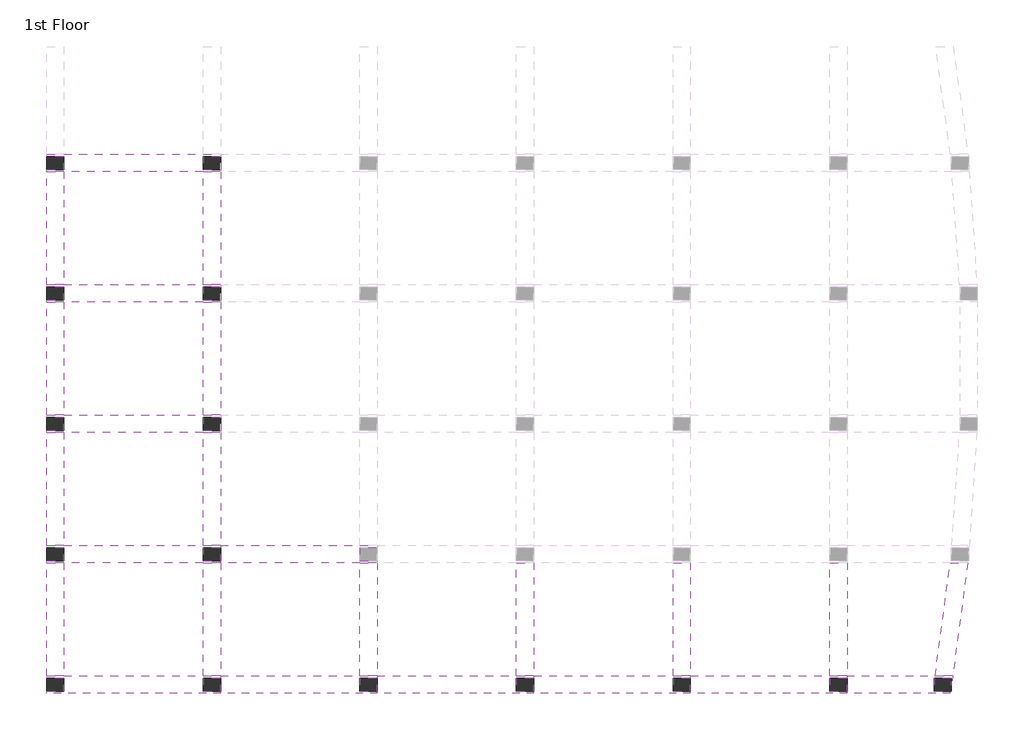
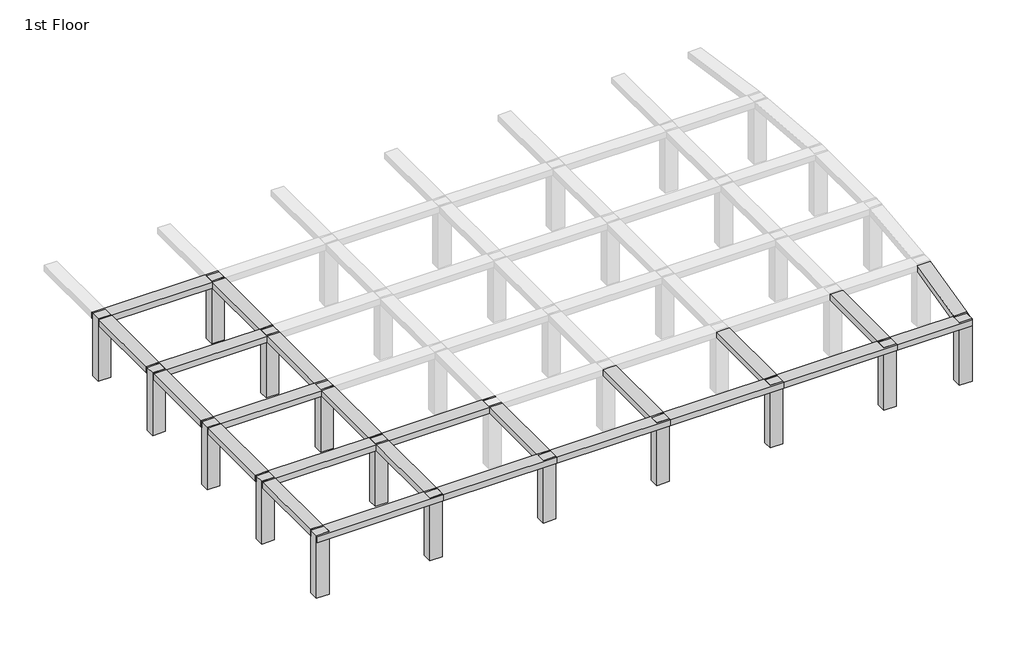
# One storey, part 1 of 3: 24 beams, 15 columns.
"""IFC4 building model written with IfcOpenShell, lengths in millimetres."""

from ifc_helpers import new_model, si_unit, frame, origin, place, context, project, spatial, polyline, outline, extrude, faceted_brep, element, save

model = new_model("IFC4")

# Units and contexts
model_context = context("Model", 3, world=origin())
ifc_project = project(units=[si_unit("LENGTHUNIT", "METRE", prefix="MILLI")], contexts=[model_context])

# Site, building, storey
site = spatial("IfcSite", under=ifc_project)
building = spatial("IfcBuilding", under=site)
storey = spatial("IfcBuildingStorey", under=building, Name="1st Floor", Elevation=3200.4)

# Beams
placement = place(None, origin())
element("IfcBeam", 1, ObjectType="Concrete-Rectangular Beam : 2' x2'", at=placement, inside=storey, context=model_context, shape_type="Brep", body=[
    faceted_brep([(-16619.274232, -2891.2168778, 6400.8), (-17228.874232, -2891.2168778, 6400.8), (-22105.674232, -2891.2168778, 6400.8), (-22715.274232, -2891.2168778, 6400.8), (-22715.274232, -2967.4168778, 6400.8), (-22105.674232, -2967.4168778, 6400.8), (-22105.674232, -3424.6168778, 6400.8), (-22715.274232, -3424.6168778, 6400.8), (-22715.274232, -3500.8168778, 6400.8), (-16619.274232, -3500.8168778, 6400.8), (-16619.274232, -3424.6168778, 6400.8), (-17228.874232, -3424.6168778, 6400.8), (-17228.874232, -2967.4168778, 6400.8), (-16619.274232, -2967.4168778, 6400.8), (-22715.274232, -3500.8168778, 6096.0), (-16619.274232, -3500.8168778, 6096.0), (-22715.274232, -3424.6168778, 6096.0), (-22105.674232, -3424.6168778, 6096.0), (-22105.674232, -2967.4168778, 6096.0), (-22715.274232, -2967.4168778, 6096.0), (-22715.274232, -2891.2168778, 6096.0), (-22105.674232, -2891.2168778, 6096.0), (-17228.874232, -2891.2168778, 6096.0), (-16619.274232, -2891.2168778, 6096.0), (-16619.274232, -2967.4168778, 6096.0), (-17228.874232, -2967.4168778, 6096.0), (-17228.874232, -3424.6168778, 6096.0), (-16619.274232, -3424.6168778, 6096.0)], [[[0, 1, 2, 3, 4, 5, 6, 7, 8, 9, 10, 11, 12, 13]], [[8, 14, 15, 9]], [[15, 14, 16, 17, 18, 19, 20, 21, 22, 23, 24, 25, 26, 27]], [[20, 3, 2, 1, 0, 23, 22, 21]], [[14, 8, 7, 16]], [[9, 15, 27, 10]], [[17, 6, 5, 18]], [[6, 17, 16, 7]], [[18, 5, 4, 19]], [[3, 20, 19, 4]], [[26, 11, 10, 27]], [[11, 26, 25, 12]], [[12, 25, 24, 13]], [[23, 0, 13, 24]]]),
])
element("IfcBeam", 2, ObjectType="Concrete-Rectangular Beam : 2' x2'", at=placement, inside=storey, context=model_context, shape_type="Brep", body=[
    faceted_brep([(-16619.274232, -2891.2168778, 6400.8), (-16619.274232, -2967.4168778, 6400.8), (-16619.274232, -3424.6168778, 6400.8), (-16619.274232, -3500.8168778, 6400.8), (-11132.874232, -3500.8168778, 6400.8), (-11132.874232, -3424.6168778, 6400.8), (-11742.474232, -3424.6168778, 6400.8), (-11742.474232, -2967.4168778, 6400.8), (-11132.874232, -2967.4168778, 6400.8), (-11132.874232, -2891.2168778, 6400.8), (-11742.474232, -2891.2168778, 6400.8), (-11132.874232, -3500.8168778, 6096.0), (-16619.274232, -3500.8168778, 6096.0), (-16619.274232, -3424.6168778, 6096.0), (-16619.274232, -2967.4168778, 6096.0), (-16619.274232, -2891.2168778, 6096.0), (-11742.474232, -2891.2168778, 6096.0), (-11132.874232, -2891.2168778, 6096.0), (-11132.874232, -2967.4168778, 6096.0), (-11742.474232, -2967.4168778, 6096.0), (-11742.474232, -3424.6168778, 6096.0), (-11132.874232, -3424.6168778, 6096.0)], [[[0, 1, 2, 3, 4, 5, 6, 7, 8, 9, 10]], [[11, 4, 3, 12]], [[12, 13, 14, 15, 16, 17, 18, 19, 20, 21, 11]], [[15, 0, 10, 9, 17, 16]], [[3, 2, 1, 0, 15, 14, 13, 12]], [[4, 11, 21, 5]], [[20, 6, 5, 21]], [[6, 20, 19, 7]], [[7, 19, 18, 8]], [[17, 9, 8, 18]]]),
])
element("IfcBeam", 3, ObjectType="Concrete-Rectangular Beam : 2' x2'", at=placement, inside=storey, context=model_context, shape_type="Brep", body=[
    faceted_brep([(-5646.474232, -2891.2168778, 6400.8), (-6256.074232, -2891.2168778, 6400.8), (-11132.874232, -2891.2168778, 6400.8), (-11132.874232, -2967.4168778, 6400.8), (-11132.874232, -3424.6168778, 6400.8), (-11132.874232, -3500.8168778, 6400.8), (-5646.474232, -3500.8168778, 6400.8), (-5646.474232, -3424.6168778, 6400.8), (-6256.074232, -3424.6168778, 6400.8), (-6256.074232, -2967.4168778, 6400.8), (-5646.474232, -2967.4168778, 6400.8), (-5646.474232, -3500.8168778, 6096.0), (-11132.874232, -3500.8168778, 6096.0), (-11132.874232, -3424.6168778, 6096.0), (-11132.874232, -2967.4168778, 6096.0), (-11132.874232, -2891.2168778, 6096.0), (-6256.074232, -2891.2168778, 6096.0), (-5646.474232, -2891.2168778, 6096.0), (-5646.474232, -2967.4168778, 6096.0), (-6256.074232, -2967.4168778, 6096.0), (-6256.074232, -3424.6168778, 6096.0), (-5646.474232, -3424.6168778, 6096.0)], [[[0, 1, 2, 3, 4, 5, 6, 7, 8, 9, 10]], [[11, 6, 5, 12]], [[11, 12, 13, 14, 15, 16, 17, 18, 19, 20, 21]], [[0, 17, 16, 15, 2, 1]], [[6, 11, 21, 7]], [[5, 4, 3, 2, 15, 14, 13, 12]], [[20, 8, 7, 21]], [[8, 20, 19, 9]], [[9, 19, 18, 10]], [[17, 0, 10, 18]]]),
])
element("IfcBeam", 4, ObjectType="Concrete-Rectangular Beam : 2' x2'", at=placement, inside=storey, context=model_context, shape_type="Brep", body=[
    faceted_brep([(-5646.474232, -2891.2168778, 6400.8), (-5646.474232, -2967.4168778, 6400.8), (-5646.474232, -3424.6168778, 6400.8), (-5646.474232, -3500.8168778, 6400.8), (-160.074232, -3500.8168778, 6400.8), (-160.074232, -3424.6168778, 6400.8), (-769.674232, -3424.6168778, 6400.8), (-769.674232, -2967.4168778, 6400.8), (-160.074232, -2967.4168778, 6400.8), (-160.074232, -2891.2168778, 6400.8), (-769.674232, -2891.2168778, 6400.8), (-160.074232, -3500.8168778, 6096.0), (-5646.474232, -3500.8168778, 6096.0), (-5646.474232, -3424.6168778, 6096.0), (-5646.474232, -2967.4168778, 6096.0), (-5646.474232, -2891.2168778, 6096.0), (-769.674232, -2891.2168778, 6096.0), (-160.074232, -2891.2168778, 6096.0), (-160.074232, -2967.4168778, 6096.0), (-769.674232, -2967.4168778, 6096.0), (-769.674232, -3424.6168778, 6096.0), (-160.074232, -3424.6168778, 6096.0)], [[[0, 1, 2, 3, 4, 5, 6, 7, 8, 9, 10]], [[11, 4, 3, 12]], [[12, 13, 14, 15, 16, 17, 18, 19, 20, 21, 11]], [[15, 0, 10, 9, 17, 16]], [[3, 2, 1, 0, 15, 14, 13, 12]], [[4, 11, 21, 5]], [[20, 6, 5, 21]], [[6, 20, 19, 7]], [[7, 19, 18, 8]], [[17, 9, 8, 18]]]),
])
element("IfcBeam", 5, ObjectType="Concrete-Rectangular Beam : 2' x2'", at=placement, inside=storey, context=model_context, shape_type="Brep", body=[
    faceted_brep([(-160.074232, -2891.2168778, 6400.8), (-160.074232, -2967.4168778, 6400.8), (-160.074232, -3424.6168778, 6400.8), (-160.074232, -3500.8168778, 6400.8), (5326.325768, -3500.8168778, 6400.8), (5326.325768, -3424.6168778, 6400.8), (4716.725768, -3424.6168778, 6400.8), (4716.725768, -2967.4168778, 6400.8), (5326.325768, -2967.4168778, 6400.8), (5326.325768, -2891.2168778, 6400.8), (4716.725768, -2891.2168778, 6400.8), (5326.325768, -3500.8168778, 6096.0), (-160.074232, -3500.8168778, 6096.0), (-160.074232, -3424.6168778, 6096.0), (-160.074232, -2967.4168778, 6096.0), (-160.074232, -2891.2168778, 6096.0), (4716.725768, -2891.2168778, 6096.0), (5326.325768, -2891.2168778, 6096.0), (5326.325768, -2967.4168778, 6096.0), (4716.725768, -2967.4168778, 6096.0), (4716.725768, -3424.6168778, 6096.0), (5326.325768, -3424.6168778, 6096.0)], [[[0, 1, 2, 3, 4, 5, 6, 7, 8, 9, 10]], [[11, 4, 3, 12]], [[12, 13, 14, 15, 16, 17, 18, 19, 20, 21, 11]], [[15, 0, 10, 9, 17, 16]], [[3, 2, 1, 0, 15, 14, 13, 12]], [[4, 11, 21, 5]], [[20, 6, 5, 21]], [[6, 20, 19, 7]], [[7, 19, 18, 8]], [[17, 9, 8, 18]]]),
])
element("IfcBeam", 6, ObjectType="Concrete-Rectangular Beam : 2' x2'", at=placement, inside=storey, context=model_context, shape_type="Brep", body=[
    faceted_brep([(9027.2344863, -2891.2168778, 6400.8), (8412.2463849, -2891.2168778, 6400.8), (5326.325768, -2891.2168778, 6400.8), (5326.325768, -2967.4168778, 6400.8), (5326.325768, -3424.6168778, 6400.8), (5326.325768, -3500.8168778, 6400.8), (8946.005151, -3500.8168778, 6400.8), (8956.158818, -3424.6168778, 6400.8), (8374.325768, -3424.6168778, 6400.8), (8374.325768, -2967.4168778, 6400.8), (8983.925768, -2967.4168778, 6400.8), (8983.925768, -3216.2348608, 6400.8), (8946.005151, -3500.8168778, 6096.0), (5326.325768, -3500.8168778, 6096.0), (5326.325768, -3424.6168778, 6096.0), (5326.325768, -2967.4168778, 6096.0), (5326.325768, -2891.2168778, 6096.0), (8412.2463849, -2891.2168778, 6096.0), (9027.2344863, -2891.2168778, 6096.0), (8983.925768, -3216.2348608, 6096.0), (8983.925768, -2967.4168778, 6096.0), (8374.325768, -2967.4168778, 6096.0), (8374.325768, -3424.6168778, 6096.0), (8956.158818, -3424.6168778, 6096.0)], [[[0, 1, 2, 3, 4, 5, 6, 7, 8, 9, 10, 11]], [[12, 6, 5, 13]], [[12, 13, 14, 15, 16, 17, 18, 19, 20, 21, 22, 23]], [[0, 18, 17, 16, 2, 1]], [[6, 12, 23, 7]], [[5, 4, 3, 2, 16, 15, 14, 13]], [[10, 20, 19, 11]], [[22, 8, 7, 23]], [[8, 22, 21, 9]], [[9, 21, 20, 10]], [[18, 0, 11, 19]]]),
])
element("IfcBeam", 7, ObjectType="Concrete-Rectangular Beam : 2' x2'", at=placement, inside=storey, context=model_context, shape_type="Brep", body=[
    faceted_brep([(-16619.274232, 1680.7831222, 6400.8), (-17228.874232, 1680.7831222, 6400.8), (-22105.674232, 1680.7831222, 6400.8), (-22715.274232, 1680.7831222, 6400.8), (-22715.274232, 1604.5831222, 6400.8), (-22105.674232, 1604.5831222, 6400.8), (-22105.674232, 1147.3831222, 6400.8), (-22715.274232, 1147.3831222, 6400.8), (-22715.274232, 1071.1831222, 6400.8), (-22105.674232, 1071.1831222, 6400.8), (-17228.874232, 1071.1831222, 6400.8), (-16619.274232, 1071.1831222, 6400.8), (-16619.274232, 1147.3831222, 6400.8), (-17228.874232, 1147.3831222, 6400.8), (-17228.874232, 1604.5831222, 6400.8), (-16619.274232, 1604.5831222, 6400.8), (-22715.274232, 1071.1831222, 6096.0), (-22105.674232, 1071.1831222, 6096.0), (-17228.874232, 1071.1831222, 6096.0), (-16619.274232, 1071.1831222, 6096.0), (-22715.274232, 1147.3831222, 6096.0), (-22105.674232, 1147.3831222, 6096.0), (-22105.674232, 1604.5831222, 6096.0), (-22715.274232, 1604.5831222, 6096.0), (-22715.274232, 1680.7831222, 6096.0), (-22105.674232, 1680.7831222, 6096.0), (-17228.874232, 1680.7831222, 6096.0), (-16619.274232, 1680.7831222, 6096.0), (-16619.274232, 1604.5831222, 6096.0), (-17228.874232, 1604.5831222, 6096.0), (-17228.874232, 1147.3831222, 6096.0), (-16619.274232, 1147.3831222, 6096.0)], [[[0, 1, 2, 3, 4, 5, 6, 7, 8, 9, 10, 11, 12, 13, 14, 15]], [[8, 16, 17, 18, 19, 11, 10, 9]], [[19, 18, 17, 16, 20, 21, 22, 23, 24, 25, 26, 27, 28, 29, 30, 31]], [[24, 3, 2, 1, 0, 27, 26, 25]], [[16, 8, 7, 20]], [[11, 19, 31, 12]], [[21, 6, 5, 22]], [[6, 21, 20, 7]], [[22, 5, 4, 23]], [[3, 24, 23, 4]], [[30, 13, 12, 31]], [[13, 30, 29, 14]], [[14, 29, 28, 15]], [[27, 0, 15, 28]]]),
])
element("IfcBeam", 8, ObjectType="Concrete-Rectangular Beam : 2' x2'", at=placement, inside=storey, context=model_context, shape_type="Brep", body=[
    faceted_brep([(-16619.274232, 1680.7831222, 6400.8), (-16619.274232, 1604.5831222, 6400.8), (-16619.274232, 1147.3831222, 6400.8), (-16619.274232, 1071.1831222, 6400.8), (-11742.474232, 1071.1831222, 6400.8), (-11132.874232, 1071.1831222, 6400.8), (-11132.874232, 1147.3831222, 6400.8), (-11742.474232, 1147.3831222, 6400.8), (-11742.474232, 1604.5831222, 6400.8), (-11132.874232, 1604.5831222, 6400.8), (-11132.874232, 1680.7831222, 6400.8), (-11742.474232, 1680.7831222, 6400.8), (-16619.274232, 1071.1831222, 6096.0), (-11742.474232, 1071.1831222, 6096.0), (-11132.874232, 1071.1831222, 6096.0), (-16619.274232, 1147.3831222, 6096.0), (-16619.274232, 1604.5831222, 6096.0), (-16619.274232, 1680.7831222, 6096.0), (-11742.474232, 1680.7831222, 6096.0), (-11132.874232, 1680.7831222, 6096.0), (-11132.874232, 1604.5831222, 6096.0), (-11742.474232, 1604.5831222, 6096.0), (-11742.474232, 1147.3831222, 6096.0), (-11132.874232, 1147.3831222, 6096.0)], [[[0, 1, 2, 3, 4, 5, 6, 7, 8, 9, 10, 11]], [[3, 12, 13, 14, 5, 4]], [[12, 15, 16, 17, 18, 19, 20, 21, 22, 23, 14, 13]], [[10, 19, 18, 17, 0, 11]], [[3, 2, 1, 0, 17, 16, 15, 12]], [[5, 14, 23, 6]], [[22, 7, 6, 23]], [[7, 22, 21, 8]], [[8, 21, 20, 9]], [[19, 10, 9, 20]]]),
])
element("IfcBeam", 9, ObjectType="Concrete-Rectangular Beam : 2' x2'", at=placement, inside=storey, context=model_context, shape_type="Brep", body=[
    faceted_brep([(-16619.274232, 6252.7831222, 6400.8), (-17228.874232, 6252.7831222, 6400.8), (-22105.674232, 6252.7831222, 6400.8), (-22715.274232, 6252.7831222, 6400.8), (-22715.274232, 6176.5831222, 6400.8), (-22105.674232, 6176.5831222, 6400.8), (-22105.674232, 5719.3831222, 6400.8), (-22715.274232, 5719.3831222, 6400.8), (-22715.274232, 5643.1831222, 6400.8), (-22105.674232, 5643.1831222, 6400.8), (-17228.874232, 5643.1831222, 6400.8), (-16619.274232, 5643.1831222, 6400.8), (-16619.274232, 5719.3831222, 6400.8), (-17228.874232, 5719.3831222, 6400.8), (-17228.874232, 6176.5831222, 6400.8), (-16619.274232, 6176.5831222, 6400.8), (-22715.274232, 5643.1831222, 6096.0), (-22105.674232, 5643.1831222, 6096.0), (-17228.874232, 5643.1831222, 6096.0), (-16619.274232, 5643.1831222, 6096.0), (-22715.274232, 5719.3831222, 6096.0), (-22105.674232, 5719.3831222, 6096.0), (-22105.674232, 6176.5831222, 6096.0), (-22715.274232, 6176.5831222, 6096.0), (-22715.274232, 6252.7831222, 6096.0), (-22105.674232, 6252.7831222, 6096.0), (-17228.874232, 6252.7831222, 6096.0), (-16619.274232, 6252.7831222, 6096.0), (-16619.274232, 6176.5831222, 6096.0), (-17228.874232, 6176.5831222, 6096.0), (-17228.874232, 5719.3831222, 6096.0), (-16619.274232, 5719.3831222, 6096.0)], [[[0, 1, 2, 3, 4, 5, 6, 7, 8, 9, 10, 11, 12, 13, 14, 15]], [[8, 16, 17, 18, 19, 11, 10, 9]], [[19, 18, 17, 16, 20, 21, 22, 23, 24, 25, 26, 27, 28, 29, 30, 31]], [[24, 3, 2, 1, 0, 27, 26, 25]], [[16, 8, 7, 20]], [[11, 19, 31, 12]], [[21, 6, 5, 22]], [[6, 21, 20, 7]], [[22, 5, 4, 23]], [[3, 24, 23, 4]], [[30, 13, 12, 31]], [[13, 30, 29, 14]], [[14, 29, 28, 15]], [[27, 0, 15, 28]]]),
])
element("IfcBeam", 10, ObjectType="Concrete-Rectangular Beam : 2' x2'", at=placement, inside=storey, context=model_context, shape_type="Brep", body=[
    faceted_brep([(-16619.274232, 10824.7831222, 6400.8), (-17228.874232, 10824.7831222, 6400.8), (-22105.674232, 10824.7831222, 6400.8), (-22715.274232, 10824.7831222, 6400.8), (-22715.274232, 10748.5831222, 6400.8), (-22105.674232, 10748.5831222, 6400.8), (-22105.674232, 10291.3831222, 6400.8), (-22715.274232, 10291.3831222, 6400.8), (-22715.274232, 10215.1831222, 6400.8), (-22105.674232, 10215.1831222, 6400.8), (-17228.874232, 10215.1831222, 6400.8), (-16619.274232, 10215.1831222, 6400.8), (-16619.274232, 10291.3831222, 6400.8), (-17228.874232, 10291.3831222, 6400.8), (-17228.874232, 10748.5831222, 6400.8), (-16619.274232, 10748.5831222, 6400.8), (-22715.274232, 10215.1831222, 6096.0), (-22105.674232, 10215.1831222, 6096.0), (-17228.874232, 10215.1831222, 6096.0), (-16619.274232, 10215.1831222, 6096.0), (-22715.274232, 10291.3831222, 6096.0), (-22105.674232, 10291.3831222, 6096.0), (-22105.674232, 10748.5831222, 6096.0), (-22715.274232, 10748.5831222, 6096.0), (-22715.274232, 10824.7831222, 6096.0), (-22105.674232, 10824.7831222, 6096.0), (-17228.874232, 10824.7831222, 6096.0), (-16619.274232, 10824.7831222, 6096.0), (-16619.274232, 10748.5831222, 6096.0), (-17228.874232, 10748.5831222, 6096.0), (-17228.874232, 10291.3831222, 6096.0), (-16619.274232, 10291.3831222, 6096.0)], [[[0, 1, 2, 3, 4, 5, 6, 7, 8, 9, 10, 11, 12, 13, 14, 15]], [[8, 16, 17, 18, 19, 11, 10, 9]], [[19, 18, 17, 16, 20, 21, 22, 23, 24, 25, 26, 27, 28, 29, 30, 31]], [[24, 3, 2, 1, 0, 27, 26, 25]], [[16, 8, 7, 20]], [[11, 19, 31, 12]], [[21, 6, 5, 22]], [[6, 21, 20, 7]], [[22, 5, 4, 23]], [[3, 24, 23, 4]], [[30, 13, 12, 31]], [[13, 30, 29, 14]], [[14, 29, 28, 15]], [[27, 0, 15, 28]]]),
])
element("IfcBeam", 11, ObjectType="Concrete-Rectangular Beam : 2' x2'", at=placement, inside=storey, context=model_context, shape_type="Brep", body=[
    faceted_brep([(-16619.274232, 15396.7831222, 6400.8), (-17228.874232, 15396.7831222, 6400.8), (-22105.674232, 15396.7831222, 6400.8), (-22715.274232, 15396.7831222, 6400.8), (-22715.274232, 15320.5831222, 6400.8), (-22105.674232, 15320.5831222, 6400.8), (-22105.674232, 14863.3831222, 6400.8), (-22715.274232, 14863.3831222, 6400.8), (-22715.274232, 14787.1831222, 6400.8), (-22105.674232, 14787.1831222, 6400.8), (-17228.874232, 14787.1831222, 6400.8), (-16619.274232, 14787.1831222, 6400.8), (-16619.274232, 14863.3831222, 6400.8), (-17228.874232, 14863.3831222, 6400.8), (-17228.874232, 15320.5831222, 6400.8), (-16619.274232, 15320.5831222, 6400.8), (-22715.274232, 14787.1831222, 6096.0), (-22105.674232, 14787.1831222, 6096.0), (-17228.874232, 14787.1831222, 6096.0), (-16619.274232, 14787.1831222, 6096.0), (-22715.274232, 14863.3831222, 6096.0), (-22105.674232, 14863.3831222, 6096.0), (-22105.674232, 15320.5831222, 6096.0), (-22715.274232, 15320.5831222, 6096.0), (-22715.274232, 15396.7831222, 6096.0), (-22105.674232, 15396.7831222, 6096.0), (-17228.874232, 15396.7831222, 6096.0), (-16619.274232, 15396.7831222, 6096.0), (-16619.274232, 15320.5831222, 6096.0), (-17228.874232, 15320.5831222, 6096.0), (-17228.874232, 14863.3831222, 6096.0), (-16619.274232, 14863.3831222, 6096.0)], [[[0, 1, 2, 3, 4, 5, 6, 7, 8, 9, 10, 11, 12, 13, 14, 15]], [[8, 16, 17, 18, 19, 11, 10, 9]], [[19, 18, 17, 16, 20, 21, 22, 23, 24, 25, 26, 27, 28, 29, 30, 31]], [[24, 3, 2, 1, 0, 27, 26, 25]], [[16, 8, 7, 20]], [[11, 19, 31, 12]], [[21, 6, 5, 22]], [[6, 21, 20, 7]], [[22, 5, 4, 23]], [[3, 24, 23, 4]], [[30, 13, 12, 31]], [[13, 30, 29, 14]], [[14, 29, 28, 15]], [[27, 0, 15, 28]]]),
])
element("IfcBeam", 12, ObjectType="Concrete-Rectangular Beam : 2' x2'", at=placement, inside=storey, context=model_context, shape_type="SweptSolid", body=[
    extrude(outline(polyline([(-22105.674232, -2891.2168778), (-22715.274232, -2891.2168778), (-22715.274232, 1071.1831222), (-22105.674232, 1071.1831222), (-22105.674232, -2891.2168778)])), frame((0.0, 0.0, 6096.0), z_axis=(0.0, 0.0, 1.0), x_axis=(1.0, 0.0, 0.0)), (0.0, 0.0, 1.0), 304.8),
])
element("IfcBeam", 13, ObjectType="Concrete-Rectangular Beam : 2' x2'", at=placement, inside=storey, context=model_context, shape_type="SweptSolid", body=[
    extrude(outline(polyline([(-22105.674232, 1680.7831222), (-22715.274232, 1680.7831222), (-22715.274232, 5643.1831222), (-22105.674232, 5643.1831222), (-22105.674232, 1680.7831222)])), frame((0.0, 0.0, 6096.0), z_axis=(0.0, 0.0, 1.0), x_axis=(1.0, 0.0, 0.0)), (0.0, 0.0, 1.0), 304.8),
])
element("IfcBeam", 14, ObjectType="Concrete-Rectangular Beam : 2' x2'", at=placement, inside=storey, context=model_context, shape_type="SweptSolid", body=[
    extrude(outline(polyline([(-22105.674232, 6252.7831222), (-22715.274232, 6252.7831222), (-22715.274232, 10215.1831222), (-22105.674232, 10215.1831222), (-22105.674232, 6252.7831222)])), frame((0.0, 0.0, 6096.0), z_axis=(0.0, 0.0, 1.0), x_axis=(1.0, 0.0, 0.0)), (0.0, 0.0, 1.0), 304.8),
])
element("IfcBeam", 15, ObjectType="Concrete-Rectangular Beam : 2' x2'", at=placement, inside=storey, context=model_context, shape_type="SweptSolid", body=[
    extrude(outline(polyline([(-22105.674232, 10824.7831222), (-22715.274232, 10824.7831222), (-22715.274232, 14787.1831222), (-22105.674232, 14787.1831222), (-22105.674232, 10824.7831222)])), frame((0.0, 0.0, 6096.0), z_axis=(0.0, 0.0, 1.0), x_axis=(1.0, 0.0, 0.0)), (0.0, 0.0, 1.0), 304.8),
])
element("IfcBeam", 16, ObjectType="Concrete-Rectangular Beam : 2' x2'", at=placement, inside=storey, context=model_context, shape_type="SweptSolid", body=[
    extrude(outline(polyline([(-17228.874232, 1071.1831222), (-16619.274232, 1071.1831222), (-16619.274232, -2891.2168778), (-17228.874232, -2891.2168778), (-17228.874232, 1071.1831222)])), frame((0.0, 0.0, 6096.0), z_axis=(0.0, 0.0, 1.0), x_axis=(1.0, 0.0, 0.0)), (0.0, 0.0, 1.0), 304.8),
])
element("IfcBeam", 17, ObjectType="Concrete-Rectangular Beam : 2' x2'", at=placement, inside=storey, context=model_context, shape_type="SweptSolid", body=[
    extrude(outline(polyline([(-16619.274232, 1680.7831222), (-17228.874232, 1680.7831222), (-17228.874232, 5643.1831222), (-16619.274232, 5643.1831222), (-16619.274232, 1680.7831222)])), frame((0.0, 0.0, 6096.0), z_axis=(0.0, 0.0, 1.0), x_axis=(1.0, 0.0, 0.0)), (0.0, 0.0, 1.0), 304.8),
])
element("IfcBeam", 18, ObjectType="Concrete-Rectangular Beam : 2' x2'", at=placement, inside=storey, context=model_context, shape_type="SweptSolid", body=[
    extrude(outline(polyline([(-16619.274232, 6252.7831222), (-17228.874232, 6252.7831222), (-17228.874232, 10215.1831222), (-16619.274232, 10215.1831222), (-16619.274232, 6252.7831222)])), frame((0.0, 0.0, 6096.0), z_axis=(0.0, 0.0, 1.0), x_axis=(1.0, 0.0, 0.0)), (0.0, 0.0, 1.0), 304.8),
])
element("IfcBeam", 19, ObjectType="Concrete-Rectangular Beam : 2' x2'", at=placement, inside=storey, context=model_context, shape_type="SweptSolid", body=[
    extrude(outline(polyline([(-16619.274232, 10824.7831222), (-17228.874232, 10824.7831222), (-17228.874232, 14787.1831222), (-16619.274232, 14787.1831222), (-16619.274232, 10824.7831222)])), frame((0.0, 0.0, 6096.0), z_axis=(0.0, 0.0, 1.0), x_axis=(1.0, 0.0, 0.0)), (0.0, 0.0, 1.0), 304.8),
])
element("IfcBeam", 20, ObjectType="Concrete-Rectangular Beam : 2' x2'", at=placement, inside=storey, context=model_context, shape_type="SweptSolid", body=[
    extrude(outline(polyline([(-11742.474232, 1071.1831222), (-11132.874232, 1071.1831222), (-11132.874232, -2891.2168778), (-11742.474232, -2891.2168778), (-11742.474232, 1071.1831222)])), frame((0.0, 0.0, 6096.0), z_axis=(0.0, 0.0, 1.0), x_axis=(1.0, 0.0, 0.0)), (0.0, 0.0, 1.0), 304.8),
])
element("IfcBeam", 21, ObjectType="Concrete-Rectangular Beam : 2' x2'", at=placement, inside=storey, context=model_context, shape_type="SweptSolid", body=[
    extrude(outline(polyline([(-6256.074232, 1071.1831222), (-5646.474232, 1071.1831222), (-5646.474232, -2891.2168778), (-6256.074232, -2891.2168778), (-6256.074232, 1071.1831222)])), frame((0.0, 0.0, 6096.0), z_axis=(0.0, 0.0, 1.0), x_axis=(1.0, 0.0, 0.0)), (0.0, 0.0, 1.0), 304.8),
])
element("IfcBeam", 22, ObjectType="Concrete-Rectangular Beam : 2' x2'", at=placement, inside=storey, context=model_context, shape_type="SweptSolid", body=[
    extrude(outline(polyline([(-769.674232, 1071.1831222), (-160.074232, 1071.1831222), (-160.074232, -2891.2168778), (-769.674232, -2891.2168778), (-769.674232, 1071.1831222)])), frame((0.0, 0.0, 6096.0), z_axis=(0.0, 0.0, 1.0), x_axis=(1.0, 0.0, 0.0)), (0.0, 0.0, 1.0), 304.8),
])
element("IfcBeam", 23, ObjectType="Concrete-Rectangular Beam : 2' x2'", at=placement, inside=storey, context=model_context, shape_type="SweptSolid", body=[
    extrude(outline(polyline([(4716.725768, 1071.1831222), (5326.325768, 1071.1831222), (5326.325768, -2891.2168778), (4716.725768, -2891.2168778), (4716.725768, 1071.1831222)])), frame((0.0, 0.0, 6096.0), z_axis=(0.0, 0.0, 1.0), x_axis=(1.0, 0.0, 0.0)), (0.0, 0.0, 1.0), 304.8),
])
element("IfcBeam", 24, ObjectType="Concrete-Rectangular Beam : 2' x2'", at=placement, inside=storey, context=model_context, shape_type="SweptSolid", body=[
    extrude(outline(polyline([(8940.2370643, 1071.1831222), (9555.2251658, 1071.1831222), (9027.2344863, -2891.2168778), (8412.2463849, -2891.2168778), (8940.2370643, 1071.1831222)])), frame((0.0, 0.0, 6096.0), z_axis=(0.0, 0.0, 1.0), x_axis=(1.0, 0.0, 0.0)), (0.0, 0.0, 1.0), 304.8),
])

# Columns
element("IfcColumn", 25, ObjectType="Concrete-Rectangular-Column : 12 x 18", at=placement, inside=storey, context=model_context, shape_type="SweptSolid", body=[
    extrude(outline(polyline([(-22105.674232, -2967.4168778), (-22105.674232, -3424.6168778), (-22715.274232, -3424.6168778), (-22715.274232, -2967.4168778), (-22105.674232, -2967.4168778)])), frame((0.0, 0.0, 3200.4), z_axis=(0.0, 0.0, 1.0), x_axis=(1.0, 0.0, 0.0)), (0.0, 0.0, 1.0), 3200.4),
])
element("IfcColumn", 26, ObjectType="Concrete-Rectangular-Column : 12 x 18", at=placement, inside=storey, context=model_context, shape_type="SweptSolid", body=[
    extrude(outline(polyline([(-16619.274232, -2967.4168778), (-16619.274232, -3424.6168778), (-17228.874232, -3424.6168778), (-17228.874232, -2967.4168778), (-16619.274232, -2967.4168778)])), frame((0.0, 0.0, 3200.4), z_axis=(0.0, 0.0, 1.0), x_axis=(1.0, 0.0, 0.0)), (0.0, 0.0, 1.0), 3200.4),
])
element("IfcColumn", 27, ObjectType="Concrete-Rectangular-Column : 12 x 18", at=placement, inside=storey, context=model_context, shape_type="SweptSolid", body=[
    extrude(outline(polyline([(-11132.874232, -2967.4168778), (-11132.874232, -3424.6168778), (-11742.474232, -3424.6168778), (-11742.474232, -2967.4168778), (-11132.874232, -2967.4168778)])), frame((0.0, 0.0, 3200.4), z_axis=(0.0, 0.0, 1.0), x_axis=(1.0, 0.0, 0.0)), (0.0, 0.0, 1.0), 3200.4),
])
element("IfcColumn", 28, ObjectType="Concrete-Rectangular-Column : 12 x 18", at=placement, inside=storey, context=model_context, shape_type="SweptSolid", body=[
    extrude(outline(polyline([(-5646.474232, -2967.4168778), (-5646.474232, -3424.6168778), (-6256.074232, -3424.6168778), (-6256.074232, -2967.4168778), (-5646.474232, -2967.4168778)])), frame((0.0, 0.0, 3200.4), z_axis=(0.0, 0.0, 1.0), x_axis=(1.0, 0.0, 0.0)), (0.0, 0.0, 1.0), 3200.4),
])
element("IfcColumn", 29, ObjectType="Concrete-Rectangular-Column : 12 x 18", at=placement, inside=storey, context=model_context, shape_type="SweptSolid", body=[
    extrude(outline(polyline([(-160.074232, -2967.4168778), (-160.074232, -3424.6168778), (-769.674232, -3424.6168778), (-769.674232, -2967.4168778), (-160.074232, -2967.4168778)])), frame((0.0, 0.0, 3200.4), z_axis=(0.0, 0.0, 1.0), x_axis=(1.0, 0.0, 0.0)), (0.0, 0.0, 1.0), 3200.4),
])
element("IfcColumn", 30, ObjectType="Concrete-Rectangular-Column : 12 x 18", at=placement, inside=storey, context=model_context, shape_type="SweptSolid", body=[
    extrude(outline(polyline([(5326.325768, -2967.4168778), (5326.325768, -3424.6168778), (4716.725768, -3424.6168778), (4716.725768, -2967.4168778), (5326.325768, -2967.4168778)])), frame((0.0, 0.0, 3200.4), z_axis=(0.0, 0.0, 1.0), x_axis=(1.0, 0.0, 0.0)), (0.0, 0.0, 1.0), 3200.4),
])
element("IfcColumn", 31, ObjectType="Concrete-Rectangular-Column : 12 x 18", at=placement, inside=storey, context=model_context, shape_type="SweptSolid", body=[
    extrude(outline(polyline([(8983.925768, -2967.4168778), (8983.925768, -3424.6168778), (8374.325768, -3424.6168778), (8374.325768, -2967.4168778), (8983.925768, -2967.4168778)])), frame((0.0, 0.0, 3200.4), z_axis=(0.0, 0.0, 1.0), x_axis=(1.0, 0.0, 0.0)), (0.0, 0.0, 1.0), 3200.4),
])
element("IfcColumn", 32, ObjectType="Concrete-Rectangular-Column : 12 x 18", at=placement, inside=storey, context=model_context, shape_type="SweptSolid", body=[
    extrude(outline(polyline([(-22105.674232, 1604.5831222), (-22105.674232, 1147.3831222), (-22715.274232, 1147.3831222), (-22715.274232, 1604.5831222), (-22105.674232, 1604.5831222)])), frame((0.0, 0.0, 3200.4), z_axis=(0.0, 0.0, 1.0), x_axis=(1.0, 0.0, 0.0)), (0.0, 0.0, 1.0), 3200.4),
])
element("IfcColumn", 33, ObjectType="Concrete-Rectangular-Column : 12 x 18", at=placement, inside=storey, context=model_context, shape_type="SweptSolid", body=[
    extrude(outline(polyline([(-16619.274232, 1604.5831222), (-16619.274232, 1147.3831222), (-17228.874232, 1147.3831222), (-17228.874232, 1604.5831222), (-16619.274232, 1604.5831222)])), frame((0.0, 0.0, 3200.4), z_axis=(0.0, 0.0, 1.0), x_axis=(1.0, 0.0, 0.0)), (0.0, 0.0, 1.0), 3200.4),
])
element("IfcColumn", 34, ObjectType="Concrete-Rectangular-Column : 12 x 18", at=placement, inside=storey, context=model_context, shape_type="SweptSolid", body=[
    extrude(outline(polyline([(-22105.674232, 6176.5831222), (-22105.674232, 5719.3831222), (-22715.274232, 5719.3831222), (-22715.274232, 6176.5831222), (-22105.674232, 6176.5831222)])), frame((0.0, 0.0, 3200.4), z_axis=(0.0, 0.0, 1.0), x_axis=(1.0, 0.0, 0.0)), (0.0, 0.0, 1.0), 3200.4),
])
element("IfcColumn", 35, ObjectType="Concrete-Rectangular-Column : 12 x 18", at=placement, inside=storey, context=model_context, shape_type="SweptSolid", body=[
    extrude(outline(polyline([(-16619.274232, 6176.5831222), (-16619.274232, 5719.3831222), (-17228.874232, 5719.3831222), (-17228.874232, 6176.5831222), (-16619.274232, 6176.5831222)])), frame((0.0, 0.0, 3200.4), z_axis=(0.0, 0.0, 1.0), x_axis=(1.0, 0.0, 0.0)), (0.0, 0.0, 1.0), 3200.4),
])
element("IfcColumn", 36, ObjectType="Concrete-Rectangular-Column : 12 x 18", at=placement, inside=storey, context=model_context, shape_type="SweptSolid", body=[
    extrude(outline(polyline([(-22105.674232, 10748.5831222), (-22105.674232, 10291.3831222), (-22715.274232, 10291.3831222), (-22715.274232, 10748.5831222), (-22105.674232, 10748.5831222)])), frame((0.0, 0.0, 3200.4), z_axis=(0.0, 0.0, 1.0), x_axis=(1.0, 0.0, 0.0)), (0.0, 0.0, 1.0), 3200.4),
])
element("IfcColumn", 37, ObjectType="Concrete-Rectangular-Column : 12 x 18", at=placement, inside=storey, context=model_context, shape_type="SweptSolid", body=[
    extrude(outline(polyline([(-16619.274232, 10748.5831222), (-16619.274232, 10291.3831222), (-17228.874232, 10291.3831222), (-17228.874232, 10748.5831222), (-16619.274232, 10748.5831222)])), frame((0.0, 0.0, 3200.4), z_axis=(0.0, 0.0, 1.0), x_axis=(1.0, 0.0, 0.0)), (0.0, 0.0, 1.0), 3200.4),
])
element("IfcColumn", 38, ObjectType="Concrete-Rectangular-Column : 12 x 18", at=placement, inside=storey, context=model_context, shape_type="SweptSolid", body=[
    extrude(outline(polyline([(-22105.674232, 15320.5831222), (-22105.674232, 14863.3831222), (-22715.274232, 14863.3831222), (-22715.274232, 15320.5831222), (-22105.674232, 15320.5831222)])), frame((0.0, 0.0, 3200.4), z_axis=(0.0, 0.0, 1.0), x_axis=(1.0, 0.0, 0.0)), (0.0, 0.0, 1.0), 3200.4),
])
element("IfcColumn", 39, ObjectType="Concrete-Rectangular-Column : 12 x 18", at=placement, inside=storey, context=model_context, shape_type="SweptSolid", body=[
    extrude(outline(polyline([(-16619.274232, 15320.5831222), (-16619.274232, 14863.3831222), (-17228.874232, 14863.3831222), (-17228.874232, 15320.5831222), (-16619.274232, 15320.5831222)])), frame((0.0, 0.0, 3200.4), z_axis=(0.0, 0.0, 1.0), x_axis=(1.0, 0.0, 0.0)), (0.0, 0.0, 1.0), 3200.4),
])

save(model, "model.ifc")

# Revit data of these elements
# Type "Concrete-Rectangular Beam : 2' x2'"
#   Assembly Code = "B10"
#   Length [instance default] = 5' - 0"
#   b = 2' - 0"
#   h = 1' - 0"
#   Structural Material [instance default] = Concrete, Cast-in-Place gray
# Type "Concrete-Rectangular-Column : 12 x 18"
#   Assembly Code = "B10"
#   b = 2' - 0"
#   h = 1' - 6"
#   Structural Material [instance default] = Concrete, Cast-in-Place gray
# Elements 1, 2, 3, 4, 5, 6, 7, 8, 9, 10, 11, 12, 13, 14, 15, 16, 17, 18, 19, 20, 21, 22, 23, 24 (IfcBeam, "Concrete-Rectangular Beam : 2' x2'")
#   Structural Material = Concrete, Precast (2)
#   Phase Created = New Construction
#   Materials on its faces: "Concrete, Precast (2)"
# Elements 25, 26, 27, 28, 29, 30, 31, 32, 33, 34, 35, 36, 37, 38, 39 (IfcColumn, "Concrete-Rectangular-Column : 12 x 18")
#   Phase Created = New Construction
#   Materials on its faces: "Concrete, Cast-in-Place gray"
# Materials
#   "Concrete, Cast-in-Place gray": class "Concrete", colour RGB 192 192 192, transparency 0, Description = "Cast-in-place concrete", Cost = 0
#   "Concrete, Precast (2)": class "Concrete", colour RGB 198 187 187, transparency 0, Description = "Precast concrete", Cost = 0
